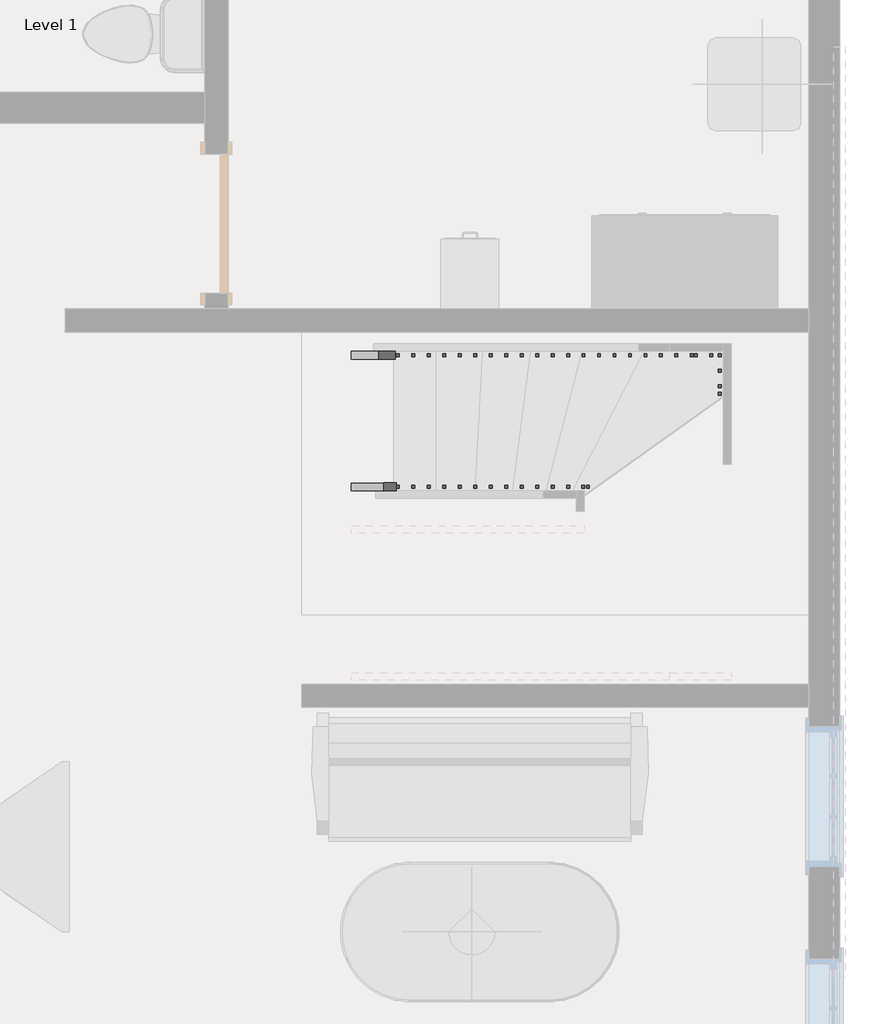
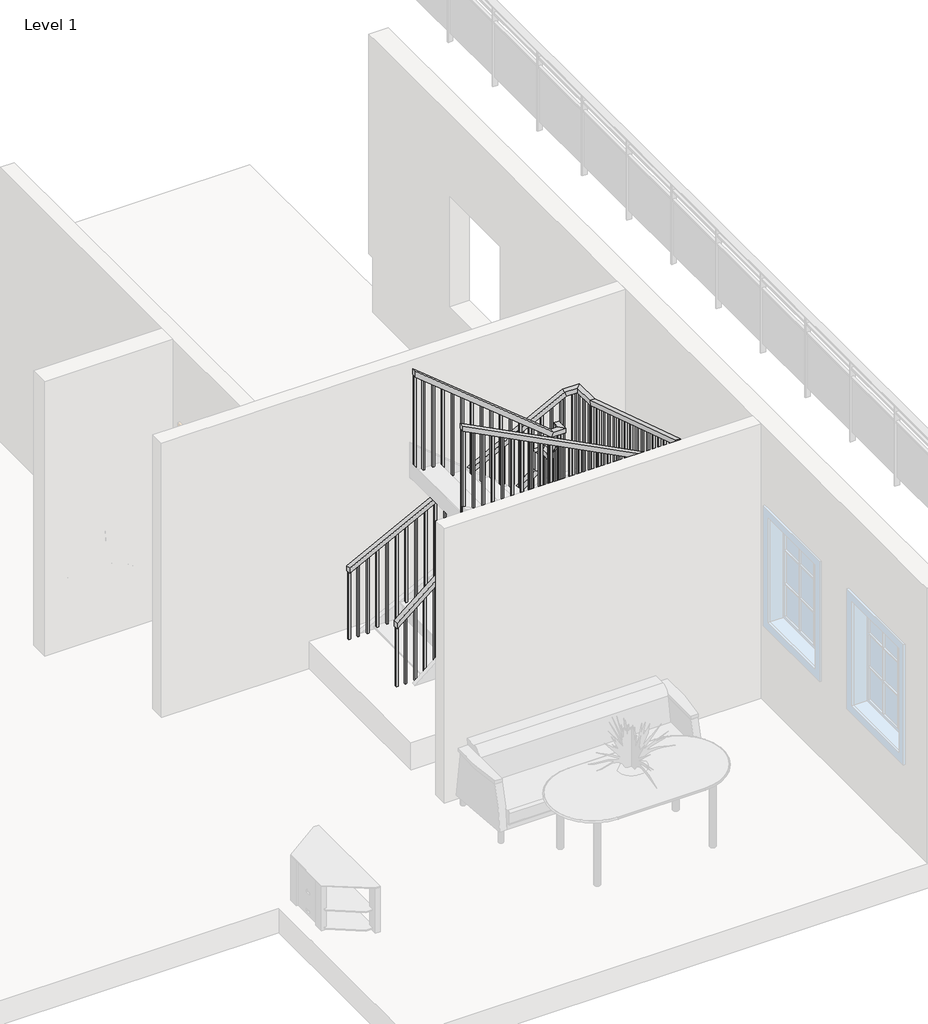
# One storey, part 2 of 4: 2 railings.
"""IFC4 building model written with IfcOpenShell, lengths in millimetres."""

from ifc_helpers import new_model, si_unit, frame, origin, place, context, project, spatial, polyline, outline, extrude, faceted_brep, element, save

model = new_model("IFC4")

# Units and contexts
model_context = context("Model", 3, world=origin())
ifc_project = project(units=[si_unit("LENGTHUNIT", "METRE", prefix="MILLI")], contexts=[model_context])

# Site, building, storey
site = spatial("IfcSite", under=ifc_project)
building = spatial("IfcBuilding", under=site)
storey = spatial("IfcBuildingStorey", under=building, Name="Level 1", Elevation=0.0)

# Railings
placement = place(None, origin())
element("IfcRailing", 1, ObjectType="Handrail - Rectangular", at=placement, inside=storey, context=model_context, shape_type="SolidModel", body=[
    faceted_brep([(-5316.1183874, 7519.8787933, 1025.2529681), (-5316.1183874, 7519.8787933, 959.7067088), (-5316.1183874, 7469.0787933, 959.7067088), (-5316.1183874, 7469.0787933, 1025.2529681), (-3864.5866955, 7519.8787933, 2208.7848338), (-3813.7866955, 7519.8787933, 2184.659247), (-3813.7866955, 7469.0787933, 2184.659247), (-3864.5866955, 7469.0787933, 2208.7848338), (-3864.5866955, 7519.8787933, 2414.6281882), (-3813.7866955, 7519.8787933, 2363.8281882), (-3813.7866955, 7469.0787933, 2363.8281882), (-3864.5866955, 7469.0787933, 2414.6281882), (-3737.5866955, 7519.8787933, 2414.6281882), (-3737.5866955, 7519.8787933, 2363.8281882), (-3788.3866955, 7469.0787933, 2363.8281882), (-3788.3866955, 7469.0787933, 2414.6281882), (-3737.5866955, 7392.8787933, 2414.6281882), (-3737.5866955, 7363.7574594, 2363.8281882), (-3788.3866955, 7363.7574594, 2363.8281882), (-3788.3866955, 7392.8787933, 2414.6281882), (-3737.5866955, 7265.8787933, 2631.5051451), (-3737.5866955, 7215.0787933, 2617.7256424), (-3788.3866955, 7215.0787933, 2617.7256424), (-3788.3866955, 7265.8787933, 2631.5051451), (-3737.5866955, 7265.8787933, 2837.3484995), (-3737.5866955, 7215.0787933, 2786.5484995), (-3788.3866955, 7215.0787933, 2786.5484995), (-3788.3866955, 7265.8787933, 2837.3484995), (-3737.5866955, 7138.8787933, 2837.3484995), (-3737.5866955, 7138.8787933, 2786.5484995), (-3788.3866955, 7189.6787933, 2786.5484995), (-3788.3866955, 7189.6787933, 2837.3484995), (-3864.5866955, 7138.8787933, 2837.3484995), (-3882.6721086, 7138.8787933, 2786.5484995), (-3882.6721086, 7189.6787933, 2786.5484995), (-3864.5866955, 7189.6787933, 2837.3484995), (-5316.1183874, 7138.8787933, 4020.8803652), (-5316.1183874, 7189.6787933, 4020.8803652), (-5316.1183874, 7189.6787933, 3955.3341059), (-5316.1183874, 7138.8787933, 3955.3341059)], [[[0, 1, 2, 3]], [[1, 0, 4, 5]], [[2, 1, 5, 6]], [[3, 2, 6, 7]], [[0, 3, 7, 4]], [[5, 4, 8, 9]], [[6, 5, 9, 10]], [[7, 6, 10, 11]], [[4, 7, 11, 8]], [[9, 8, 12, 13]], [[10, 9, 13, 14]], [[11, 10, 14, 15]], [[8, 11, 15, 12]], [[13, 12, 16, 17]], [[14, 13, 17, 18]], [[15, 14, 18, 19]], [[12, 15, 19, 16]], [[17, 16, 20, 21]], [[18, 17, 21, 22]], [[19, 18, 22, 23]], [[16, 19, 23, 20]], [[21, 20, 24, 25]], [[22, 21, 25, 26]], [[23, 22, 26, 27]], [[20, 23, 27, 24]], [[25, 24, 28, 29]], [[26, 25, 29, 30]], [[27, 26, 30, 31]], [[24, 27, 31, 28]], [[29, 28, 32, 33]], [[30, 29, 33, 34]], [[31, 30, 34, 35]], [[28, 31, 35, 32]], [[36, 37, 38, 39]], [[33, 32, 36, 39]], [[34, 33, 39, 38]], [[35, 34, 38, 37]], [[32, 35, 37, 36]]]),
    extrude(outline(polyline([(3866.2231262, -5206.8290519), (3881.7558784, -5225.8790519), (2878.6666667, -5225.8790519), (2878.6666667, -5206.8290519), (3866.2231262, -5206.8290519)])), frame((0.0, 7154.7537933, 0.0), z_axis=(0.0, 1.0, 0.0), x_axis=(0.0, 0.0, 1.0)), (0.0, 0.0, 1.0), 19.05),
    extrude(outline(polyline([(3783.3817813, -5105.2290519), (3798.9145334, -5124.2790519), (2878.6666667, -5124.2790519), (2878.6666667, -5105.2290519), (3783.3817813, -5105.2290519)])), frame((0.0, 7154.7537933, 0.0), z_axis=(0.0, 1.0, 0.0), x_axis=(0.0, 0.0, 1.0)), (0.0, 0.0, 1.0), 19.05),
    extrude(outline(polyline([(3700.5404364, -5003.6290519), (3716.0731885, -5022.6790519), (2709.3333333, -5022.6790519), (2709.3333333, -5003.6290519), (3700.5404364, -5003.6290519)])), frame((0.0, 7154.7537933, 0.0), z_axis=(0.0, 1.0, 0.0), x_axis=(0.0, 0.0, 1.0)), (0.0, 0.0, 1.0), 19.05),
    extrude(outline(polyline([(3617.6990914, -4902.0290519), (3633.2318436, -4921.0790519), (2709.3333333, -4921.0790519), (2709.3333333, -4902.0290519), (3617.6990914, -4902.0290519)])), frame((0.0, 7154.7537933, 0.0), z_axis=(0.0, 1.0, 0.0), x_axis=(0.0, 0.0, 1.0)), (0.0, 0.0, 1.0), 19.05),
    extrude(outline(polyline([(3534.8577465, -4800.4290519), (3550.3904987, -4819.4790519), (2709.3333333, -4819.4790519), (2709.3333333, -4800.4290519), (3534.8577465, -4800.4290519)])), frame((0.0, 7154.7537933, 0.0), z_axis=(0.0, 1.0, 0.0), x_axis=(0.0, 0.0, 1.0)), (0.0, 0.0, 1.0), 19.05),
    extrude(outline(polyline([(3452.0164016, -4698.8290519), (3467.5491538, -4717.8790519), (2540.0, -4717.8790519), (2540.0, -4698.8290519), (3452.0164016, -4698.8290519)])), frame((0.0, 7154.7537933, 0.0), z_axis=(0.0, 1.0, 0.0), x_axis=(0.0, 0.0, 1.0)), (0.0, 0.0, 1.0), 19.05),
    extrude(outline(polyline([(3369.1750567, -4597.2290519), (3384.7078088, -4616.2790519), (2540.0, -4616.2790519), (2540.0, -4597.2290519), (3369.1750567, -4597.2290519)])), frame((0.0, 7154.7537933, 0.0), z_axis=(0.0, 1.0, 0.0), x_axis=(0.0, 0.0, 1.0)), (0.0, 0.0, 1.0), 19.05),
    extrude(outline(polyline([(3286.3337117, -4495.6290519), (3301.8664639, -4514.6790519), (2540.0, -4514.6790519), (2540.0, -4495.6290519), (3286.3337117, -4495.6290519)])), frame((0.0, 7154.7537933, 0.0), z_axis=(0.0, 1.0, 0.0), x_axis=(0.0, 0.0, 1.0)), (0.0, 0.0, 1.0), 19.05),
    extrude(outline(polyline([(3203.4923668, -4394.0290519), (3219.025119, -4413.0790519), (2370.6666667, -4413.0790519), (2370.6666667, -4394.0290519), (3203.4923668, -4394.0290519)])), frame((0.0, 7154.7537933, 0.0), z_axis=(0.0, 1.0, 0.0), x_axis=(0.0, 0.0, 1.0)), (0.0, 0.0, 1.0), 19.05),
    extrude(outline(polyline([(3120.6510219, -4292.4290519), (3136.1837741, -4311.4790519), (2370.6666667, -4311.4790519), (2370.6666667, -4292.4290519), (3120.6510219, -4292.4290519)])), frame((0.0, 7154.7537933, 0.0), z_axis=(0.0, 1.0, 0.0), x_axis=(0.0, 0.0, 1.0)), (0.0, 0.0, 1.0), 19.05),
    extrude(outline(polyline([(3037.809677, -4190.8290519), (3053.3424291, -4209.8790519), (2201.3333333, -4209.8790519), (2201.3333333, -4190.8290519), (3037.809677, -4190.8290519)])), frame((0.0, 7154.7537933, 0.0), z_axis=(0.0, 1.0, 0.0), x_axis=(0.0, 0.0, 1.0)), (0.0, 0.0, 1.0), 19.05),
    extrude(outline(polyline([(2954.9683321, -4089.2290519), (2970.5010842, -4108.2790519), (2201.3333333, -4108.2790519), (2201.3333333, -4089.2290519), (2954.9683321, -4089.2290519)])), frame((0.0, 7154.7537933, 0.0), z_axis=(0.0, 1.0, 0.0), x_axis=(0.0, 0.0, 1.0)), (0.0, 0.0, 1.0), 19.05),
    extrude(outline(polyline([(2872.1269871, -3987.6290519), (2887.6597393, -4006.6790519), (2032.0, -4006.6790519), (2032.0, -3987.6290519), (2872.1269871, -3987.6290519)])), frame((0.0, 7154.7537933, 0.0), z_axis=(0.0, 1.0, 0.0), x_axis=(0.0, 0.0, 1.0)), (0.0, 0.0, 1.0), 19.05),
    extrude(outline(polyline([(2789.2856422, -3886.0290519), (2804.8183944, -3905.0790519), (2032.0, -3905.0790519), (2032.0, -3886.0290519), (2789.2856422, -3886.0290519)])), frame((0.0, 7154.7537933, 0.0), z_axis=(0.0, 1.0, 0.0), x_axis=(0.0, 0.0, 1.0)), (0.0, 0.0, 1.0), 19.05),
    extrude(outline(polyline([(7266.9678895, 2529.115018), (7286.0178895, 2496.5834745), (7286.0178895, 1524.0), (7266.9678895, 1524.0), (7266.9678895, 2529.115018)])), frame((-3772.5116955, 0.0, 0.0), z_axis=(1.0, 0.0, 0.0), x_axis=(0.0, 1.0, 0.0)), (0.0, 0.0, 1.0), 19.05),
    extrude(outline(polyline([(7368.5678895, 2355.6134525), (7387.6178895, 2323.0819089), (7387.6178895, 1524.0), (7368.5678895, 1524.0), (7368.5678895, 2355.6134525)])), frame((-3772.5116955, 0.0, 0.0), z_axis=(1.0, 0.0, 0.0), x_axis=(0.0, 1.0, 0.0)), (0.0, 0.0, 1.0), 19.05),
    extrude(outline(polyline([(2127.2519138, -3884.1933874), (2111.7191617, -3903.2433874), (1016.0, -3903.2433874), (1016.0, -3884.1933874), (2127.2519138, -3884.1933874)])), frame((0.0, 7484.9537933, 0.0), z_axis=(0.0, 1.0, 0.0), x_axis=(0.0, 0.0, 1.0)), (0.0, 0.0, 1.0), 19.05),
    extrude(outline(polyline([(2044.4105689, -3985.7933874), (2028.8778167, -4004.8433874), (1016.0, -4004.8433874), (1016.0, -3985.7933874), (2044.4105689, -3985.7933874)])), frame((0.0, 7484.9537933, 0.0), z_axis=(0.0, 1.0, 0.0), x_axis=(0.0, 0.0, 1.0)), (0.0, 0.0, 1.0), 19.05),
    extrude(outline(polyline([(1961.569224, -4087.3933874), (1946.0364718, -4106.4433874), (846.6666667, -4106.4433874), (846.6666667, -4087.3933874), (1961.569224, -4087.3933874)])), frame((0.0, 7484.9537933, 0.0), z_axis=(0.0, 1.0, 0.0), x_axis=(0.0, 0.0, 1.0)), (0.0, 0.0, 1.0), 19.05),
    extrude(outline(polyline([(1878.7278791, -4188.9933874), (1863.1951269, -4208.0433874), (846.6666667, -4208.0433874), (846.6666667, -4188.9933874), (1878.7278791, -4188.9933874)])), frame((0.0, 7484.9537933, 0.0), z_axis=(0.0, 1.0, 0.0), x_axis=(0.0, 0.0, 1.0)), (0.0, 0.0, 1.0), 19.05),
    extrude(outline(polyline([(1795.8865341, -4290.5933874), (1780.353782, -4309.6433874), (677.3333333, -4309.6433874), (677.3333333, -4290.5933874), (1795.8865341, -4290.5933874)])), frame((0.0, 7484.9537933, 0.0), z_axis=(0.0, 1.0, 0.0), x_axis=(0.0, 0.0, 1.0)), (0.0, 0.0, 1.0), 19.05),
    extrude(outline(polyline([(1713.0451892, -4392.1933874), (1697.5124371, -4411.2433874), (677.3333333, -4411.2433874), (677.3333333, -4392.1933874), (1713.0451892, -4392.1933874)])), frame((0.0, 7484.9537933, 0.0), z_axis=(0.0, 1.0, 0.0), x_axis=(0.0, 0.0, 1.0)), (0.0, 0.0, 1.0), 19.05),
    extrude(outline(polyline([(1630.2038443, -4493.7933874), (1614.6710921, -4512.8433874), (508.0, -4512.8433874), (508.0, -4493.7933874), (1630.2038443, -4493.7933874)])), frame((0.0, 7484.9537933, 0.0), z_axis=(0.0, 1.0, 0.0), x_axis=(0.0, 0.0, 1.0)), (0.0, 0.0, 1.0), 19.05),
    extrude(outline(polyline([(1547.3624994, -4595.3933874), (1531.8297472, -4614.4433874), (508.0, -4614.4433874), (508.0, -4595.3933874), (1547.3624994, -4595.3933874)])), frame((0.0, 7484.9537933, 0.0), z_axis=(0.0, 1.0, 0.0), x_axis=(0.0, 0.0, 1.0)), (0.0, 0.0, 1.0), 19.05),
    extrude(outline(polyline([(1464.5211545, -4696.9933874), (1448.9884023, -4716.0433874), (508.0, -4716.0433874), (508.0, -4696.9933874), (1464.5211545, -4696.9933874)])), frame((0.0, 7484.9537933, 0.0), z_axis=(0.0, 1.0, 0.0), x_axis=(0.0, 0.0, 1.0)), (0.0, 0.0, 1.0), 19.05),
    extrude(outline(polyline([(1381.6798095, -4798.5933874), (1366.1470574, -4817.6433874), (338.6666667, -4817.6433874), (338.6666667, -4798.5933874), (1381.6798095, -4798.5933874)])), frame((0.0, 7484.9537933, 0.0), z_axis=(0.0, 1.0, 0.0), x_axis=(0.0, 0.0, 1.0)), (0.0, 0.0, 1.0), 19.05),
    extrude(outline(polyline([(1298.8384646, -4900.1933874), (1283.3057124, -4919.2433874), (338.6666667, -4919.2433874), (338.6666667, -4900.1933874), (1298.8384646, -4900.1933874)])), frame((0.0, 7484.9537933, 0.0), z_axis=(0.0, 1.0, 0.0), x_axis=(0.0, 0.0, 1.0)), (0.0, 0.0, 1.0), 19.05),
    extrude(outline(polyline([(1215.9971197, -5001.7933874), (1200.4643675, -5020.8433874), (338.6666667, -5020.8433874), (338.6666667, -5001.7933874), (1215.9971197, -5001.7933874)])), frame((0.0, 7484.9537933, 0.0), z_axis=(0.0, 1.0, 0.0), x_axis=(0.0, 0.0, 1.0)), (0.0, 0.0, 1.0), 19.05),
    extrude(outline(polyline([(1133.1557748, -5103.3933874), (1117.6230226, -5122.4433874), (169.3333333, -5122.4433874), (169.3333333, -5103.3933874), (1133.1557748, -5103.3933874)])), frame((0.0, 7484.9537933, 0.0), z_axis=(0.0, 1.0, 0.0), x_axis=(0.0, 0.0, 1.0)), (0.0, 0.0, 1.0), 19.05),
    extrude(outline(polyline([(1050.3144298, -5204.9933874), (1034.7816777, -5224.0433874), (169.3333333, -5224.0433874), (169.3333333, -5204.9933874), (1050.3144298, -5204.9933874)])), frame((0.0, 7484.9537933, 0.0), z_axis=(0.0, 1.0, 0.0), x_axis=(0.0, 0.0, 1.0)), (0.0, 0.0, 1.0), 19.05),
    extrude(outline(polyline([(-3784.4290519, 7173.8037933), (-3784.4290519, 7154.7537933), (-3803.4790519, 7154.7537933), (-3803.4790519, 7173.8037933), (-3784.4290519, 7173.8037933)])), frame((0.0, 0.0, 1862.6666667), z_axis=(0.0, 0.0, 1.0), x_axis=(1.0, 0.0, 0.0)), (0.0, 0.0, 1.0), 923.8818329),
    extrude(outline(polyline([(-3772.5116955, 7173.8037933), (-3753.4616955, 7173.8037933), (-3753.4616955, 7154.7537933), (-3772.5116955, 7154.7537933), (-3772.5116955, 7173.8037933)])), frame((0.0, 0.0, 1862.6666667), z_axis=(0.0, 0.0, 1.0), x_axis=(1.0, 0.0, 0.0)), (0.0, 0.0, 1.0), 923.8818329),
    extrude(outline(polyline([(-3772.5116955, 7188.589697), (-3753.4616955, 7188.589697), (-3753.4616955, 7169.539697), (-3772.5116955, 7169.539697), (-3772.5116955, 7188.589697)])), frame((0.0, 0.0, 1693.3333333), z_axis=(0.0, 0.0, 1.0), x_axis=(1.0, 0.0, 0.0)), (0.0, 0.0, 1.0), 1093.2151662),
    extrude(outline(polyline([(-3772.5116955, 7489.2178895), (-3753.4616955, 7489.2178895), (-3753.4616955, 7470.1678895), (-3772.5116955, 7470.1678895), (-3772.5116955, 7489.2178895)])), frame((0.0, 0.0, 1354.6666667), z_axis=(0.0, 0.0, 1.0), x_axis=(1.0, 0.0, 0.0)), (0.0, 0.0, 1.0), 1009.1615215),
    extrude(outline(polyline([(-3772.5116955, 7484.9537933), (-3772.5116955, 7504.0037933), (-3753.4616955, 7504.0037933), (-3753.4616955, 7484.9537933), (-3772.5116955, 7484.9537933)])), frame((0.0, 0.0, 1185.3333333), z_axis=(0.0, 0.0, 1.0), x_axis=(1.0, 0.0, 0.0)), (0.0, 0.0, 1.0), 1178.4948549),
    extrude(outline(polyline([(-3803.4790519, 7484.9537933), (-3803.4790519, 7504.0037933), (-3784.4290519, 7504.0037933), (-3784.4290519, 7484.9537933), (-3803.4790519, 7484.9537933)])), frame((0.0, 0.0, 1185.3333333), z_axis=(0.0, 0.0, 1.0), x_axis=(1.0, 0.0, 0.0)), (0.0, 0.0, 1.0), 1178.4948549),
    extrude(outline(polyline([(3939.8013537, -5297.0683874), (3955.3341059, -5316.1183874), (2878.6666667, -5316.1183874), (2878.6666667, -5297.0683874), (3939.8013537, -5297.0683874)])), frame((0.0, 7154.7537933, 0.0), z_axis=(0.0, 1.0, 0.0), x_axis=(0.0, 0.0, 1.0)), (0.0, 0.0, 1.0), 19.05),
    extrude(outline(polyline([(975.239461, -5297.0683874), (959.7067088, -5316.1183874), (169.3333333, -5316.1183874), (169.3333333, -5297.0683874), (975.239461, -5297.0683874)])), frame((0.0, 7484.9537933, 0.0), z_axis=(0.0, 1.0, 0.0), x_axis=(0.0, 0.0, 1.0)), (0.0, 0.0, 1.0), 19.05),
])
element("IfcRailing", 2, ObjectType="Handrail - Rectangular", at=placement, inside=storey, context=model_context, shape_type="SolidModel", body=[
    faceted_brep([(-5316.1183874, 8383.4787933, 1109.0771751), (-5316.1183874, 8383.4787933, 1051.9280057), (-5316.1183874, 8332.6787933, 1051.9280057), (-5316.1183874, 8332.6787933, 1109.0771751), (-3056.1365309, 8383.4787933, 2273.7644996), (-3043.8164796, 8383.4787933, 2222.9644996), (-3043.8164796, 8332.6787933, 2222.9644996), (-3056.1365309, 8332.6787933, 2273.7644996), (-2873.9866955, 8383.4787933, 2273.7644996), (-2873.9866955, 8383.4787933, 2222.9644996), (-2924.7866955, 8332.6787933, 2222.9644996), (-2924.7866955, 8332.6787933, 2273.7644996), (-2873.9866955, 8106.3248407, 2273.7644996), (-2873.9866955, 8098.3742645, 2222.9644996), (-2924.7866955, 8098.3742645, 2222.9644996), (-2924.7866955, 8106.3248407, 2273.7644996), (-2873.9866955, 6552.4327459, 2772.3688337), (-2873.9866955, 6544.4821698, 2721.5688337), (-2924.7866955, 6544.4821698, 2721.5688337), (-2924.7866955, 6552.4327459, 2772.3688337), (-2873.9866955, 6275.2787933, 2772.3688337), (-2873.9866955, 6275.2787933, 2721.5688337), (-2924.7866955, 6326.0787933, 2721.5688337), (-2924.7866955, 6326.0787933, 2772.3688337), (-3056.1365309, 6275.2787933, 2772.3688337), (-3068.4565822, 6275.2787933, 2721.5688337), (-3068.4565822, 6326.0787933, 2721.5688337), (-3056.1365309, 6326.0787933, 2772.3688337), (-5316.1183874, 6275.2787933, 3937.0561582), (-5316.1183874, 6326.0787933, 3937.0561582), (-5316.1183874, 6326.0787933, 3879.9069889), (-5316.1183874, 6275.2787933, 3879.9069889)], [[[0, 1, 2, 3]], [[1, 0, 4, 5]], [[2, 1, 5, 6]], [[3, 2, 6, 7]], [[0, 3, 7, 4]], [[5, 4, 8, 9]], [[6, 5, 9, 10]], [[7, 6, 10, 11]], [[4, 7, 11, 8]], [[9, 8, 12, 13]], [[10, 9, 13, 14]], [[11, 10, 14, 15]], [[8, 11, 15, 12]], [[13, 12, 16, 17]], [[14, 13, 17, 18]], [[15, 14, 18, 19]], [[12, 15, 19, 16]], [[17, 16, 20, 21]], [[18, 17, 21, 22]], [[19, 18, 22, 23]], [[16, 19, 23, 20]], [[21, 20, 24, 25]], [[22, 21, 25, 26]], [[23, 22, 26, 27]], [[20, 23, 27, 24]], [[28, 29, 30, 31]], [[25, 24, 28, 31]], [[26, 25, 31, 30]], [[27, 26, 30, 29]], [[24, 27, 29, 28]]]),
    extrude(outline(polyline([(3872.0443296, -5300.8615309), (2878.6666667, -5300.8615309), (2878.6666667, -5281.8115309), (3862.2268642, -5281.8115309), (3872.0443296, -5300.8615309)])), frame((0.0, 6291.1537933, 0.0), z_axis=(0.0, 1.0, 0.0), x_axis=(0.0, 0.0, 1.0)), (0.0, 0.0, 1.0), 19.05),
    extrude(outline(polyline([(3819.6845145, -5199.2615309), (2878.6666667, -5199.2615309), (2878.6666667, -5180.2115309), (3809.8670491, -5180.2115309), (3819.6845145, -5199.2615309)])), frame((0.0, 6291.1537933, 0.0), z_axis=(0.0, 1.0, 0.0), x_axis=(0.0, 0.0, 1.0)), (0.0, 0.0, 1.0), 19.05),
    extrude(outline(polyline([(3767.3246993, -5097.6615309), (2878.6666667, -5097.6615309), (2878.6666667, -5078.6115309), (3757.507234, -5078.6115309), (3767.3246993, -5097.6615309)])), frame((0.0, 6291.1537933, 0.0), z_axis=(0.0, 1.0, 0.0), x_axis=(0.0, 0.0, 1.0)), (0.0, 0.0, 1.0), 19.05),
    extrude(outline(polyline([(3714.9648842, -4996.0615309), (2709.3333333, -4996.0615309), (2709.3333333, -4977.0115309), (3705.1474189, -4977.0115309), (3714.9648842, -4996.0615309)])), frame((0.0, 6291.1537933, 0.0), z_axis=(0.0, 1.0, 0.0), x_axis=(0.0, 0.0, 1.0)), (0.0, 0.0, 1.0), 19.05),
    extrude(outline(polyline([(3662.6050691, -4894.4615309), (2709.3333333, -4894.4615309), (2709.3333333, -4875.4115309), (3652.7876038, -4875.4115309), (3662.6050691, -4894.4615309)])), frame((0.0, 6291.1537933, 0.0), z_axis=(0.0, 1.0, 0.0), x_axis=(0.0, 0.0, 1.0)), (0.0, 0.0, 1.0), 19.05),
    extrude(outline(polyline([(3610.245254, -4792.8615309), (2709.3333333, -4792.8615309), (2709.3333333, -4773.8115309), (3600.4277887, -4773.8115309), (3610.245254, -4792.8615309)])), frame((0.0, 6291.1537933, 0.0), z_axis=(0.0, 1.0, 0.0), x_axis=(0.0, 0.0, 1.0)), (0.0, 0.0, 1.0), 19.05),
    extrude(outline(polyline([(3557.8854389, -4691.2615309), (2540.0, -4691.2615309), (2540.0, -4672.2115309), (3548.0679735, -4672.2115309), (3557.8854389, -4691.2615309)])), frame((0.0, 6291.1537933, 0.0), z_axis=(0.0, 1.0, 0.0), x_axis=(0.0, 0.0, 1.0)), (0.0, 0.0, 1.0), 19.05),
    extrude(outline(polyline([(3505.5256238, -4589.6615309), (2540.0, -4589.6615309), (2540.0, -4570.6115309), (3495.7081584, -4570.6115309), (3505.5256238, -4589.6615309)])), frame((0.0, 6291.1537933, 0.0), z_axis=(0.0, 1.0, 0.0), x_axis=(0.0, 0.0, 1.0)), (0.0, 0.0, 1.0), 19.05),
    extrude(outline(polyline([(3453.1658086, -4488.0615309), (2540.0, -4488.0615309), (2540.0, -4469.0115309), (3443.3483433, -4469.0115309), (3453.1658086, -4488.0615309)])), frame((0.0, 6291.1537933, 0.0), z_axis=(0.0, 1.0, 0.0), x_axis=(0.0, 0.0, 1.0)), (0.0, 0.0, 1.0), 19.05),
    extrude(outline(polyline([(3400.8059935, -4386.4615309), (2370.6666667, -4386.4615309), (2370.6666667, -4367.4115309), (3390.9885282, -4367.4115309), (3400.8059935, -4386.4615309)])), frame((0.0, 6291.1537933, 0.0), z_axis=(0.0, 1.0, 0.0), x_axis=(0.0, 0.0, 1.0)), (0.0, 0.0, 1.0), 19.05),
    extrude(outline(polyline([(3348.4461784, -4284.8615309), (2370.6666667, -4284.8615309), (2370.6666667, -4265.8115309), (3338.6287131, -4265.8115309), (3348.4461784, -4284.8615309)])), frame((0.0, 6291.1537933, 0.0), z_axis=(0.0, 1.0, 0.0), x_axis=(0.0, 0.0, 1.0)), (0.0, 0.0, 1.0), 19.05),
    extrude(outline(polyline([(3296.0863633, -4183.2615309), (2370.6666667, -4183.2615309), (2370.6666667, -4164.2115309), (3286.268898, -4164.2115309), (3296.0863633, -4183.2615309)])), frame((0.0, 6291.1537933, 0.0), z_axis=(0.0, 1.0, 0.0), x_axis=(0.0, 0.0, 1.0)), (0.0, 0.0, 1.0), 19.05),
    extrude(outline(polyline([(3243.7265482, -4081.6615309), (2201.3333333, -4081.6615309), (2201.3333333, -4062.6115309), (3233.9090828, -4062.6115309), (3243.7265482, -4081.6615309)])), frame((0.0, 6291.1537933, 0.0), z_axis=(0.0, 1.0, 0.0), x_axis=(0.0, 0.0, 1.0)), (0.0, 0.0, 1.0), 19.05),
    extrude(outline(polyline([(3191.3667331, -3980.0615309), (2201.3333333, -3980.0615309), (2201.3333333, -3961.0115309), (3181.5492677, -3961.0115309), (3191.3667331, -3980.0615309)])), frame((0.0, 6291.1537933, 0.0), z_axis=(0.0, 1.0, 0.0), x_axis=(0.0, 0.0, 1.0)), (0.0, 0.0, 1.0), 19.05),
    extrude(outline(polyline([(3139.0069179, -3878.4615309), (2201.3333333, -3878.4615309), (2201.3333333, -3859.4115309), (3129.1894526, -3859.4115309), (3139.0069179, -3878.4615309)])), frame((0.0, 6291.1537933, 0.0), z_axis=(0.0, 1.0, 0.0), x_axis=(0.0, 0.0, 1.0)), (0.0, 0.0, 1.0), 19.05),
    extrude(outline(polyline([(3086.6471028, -3776.8615309), (2032.0, -3776.8615309), (2032.0, -3757.8115309), (3076.8296375, -3757.8115309), (3086.6471028, -3776.8615309)])), frame((0.0, 6291.1537933, 0.0), z_axis=(0.0, 1.0, 0.0), x_axis=(0.0, 0.0, 1.0)), (0.0, 0.0, 1.0), 19.05),
    extrude(outline(polyline([(3034.2872877, -3675.2615309), (2032.0, -3675.2615309), (2032.0, -3656.2115309), (3024.4698224, -3656.2115309), (3034.2872877, -3675.2615309)])), frame((0.0, 6291.1537933, 0.0), z_axis=(0.0, 1.0, 0.0), x_axis=(0.0, 0.0, 1.0)), (0.0, 0.0, 1.0), 19.05),
    extrude(outline(polyline([(2981.9274726, -3573.6615309), (2032.0, -3573.6615309), (2032.0, -3554.6115309), (2972.1100073, -3554.6115309), (2981.9274726, -3573.6615309)])), frame((0.0, 6291.1537933, 0.0), z_axis=(0.0, 1.0, 0.0), x_axis=(0.0, 0.0, 1.0)), (0.0, 0.0, 1.0), 19.05),
    extrude(outline(polyline([(2929.5676575, -3472.0615309), (2032.0, -3472.0615309), (2032.0, -3453.0115309), (2919.7501921, -3453.0115309), (2929.5676575, -3472.0615309)])), frame((0.0, 6291.1537933, 0.0), z_axis=(0.0, 1.0, 0.0), x_axis=(0.0, 0.0, 1.0)), (0.0, 0.0, 1.0), 19.05),
    extrude(outline(polyline([(2877.2078424, -3370.4615309), (1862.6666667, -3370.4615309), (1862.6666667, -3351.4115309), (2867.390377, -3351.4115309), (2877.2078424, -3370.4615309)])), frame((0.0, 6291.1537933, 0.0), z_axis=(0.0, 1.0, 0.0), x_axis=(0.0, 0.0, 1.0)), (0.0, 0.0, 1.0), 19.05),
    extrude(outline(polyline([(2824.8480272, -3268.8615309), (1862.6666667, -3268.8615309), (1862.6666667, -3249.8115309), (2815.0305619, -3249.8115309), (2824.8480272, -3268.8615309)])), frame((0.0, 6291.1537933, 0.0), z_axis=(0.0, 1.0, 0.0), x_axis=(0.0, 0.0, 1.0)), (0.0, 0.0, 1.0), 19.05),
    extrude(outline(polyline([(2772.4882121, -3167.2615309), (1862.6666667, -3167.2615309), (1862.6666667, -3148.2115309), (2762.6707468, -3148.2115309), (2772.4882121, -3167.2615309)])), frame((0.0, 6291.1537933, 0.0), z_axis=(0.0, 1.0, 0.0), x_axis=(0.0, 0.0, 1.0)), (0.0, 0.0, 1.0), 19.05),
    extrude(outline(polyline([(-2991.4616955, 6291.1537933), (-3010.5116955, 6291.1537933), (-3010.5116955, 6310.2037933), (-2991.4616955, 6310.2037933), (-2991.4616955, 6291.1537933)])), frame((0.0, 0.0, 1862.6666667), z_axis=(0.0, 0.0, 1.0), x_axis=(1.0, 0.0, 0.0)), (0.0, 0.0, 1.0), 858.902167),
    extrude(outline(polyline([(-2889.8616955, 6358.7577459), (-2889.8616955, 6339.7077459), (-2908.9116955, 6339.7077459), (-2908.9116955, 6358.7577459), (-2889.8616955, 6358.7577459)])), frame((0.0, 0.0, 1862.6666667), z_axis=(0.0, 0.0, 1.0), x_axis=(1.0, 0.0, 0.0)), (0.0, 0.0, 1.0), 858.902167),
    extrude(outline(polyline([(-2889.8616955, 6460.3577459), (-2889.8616955, 6441.3077459), (-2908.9116955, 6441.3077459), (-2908.9116955, 6460.3577459), (-2889.8616955, 6460.3577459)])), frame((0.0, 0.0, 1862.6666667), z_axis=(0.0, 0.0, 1.0), x_axis=(1.0, 0.0, 0.0)), (0.0, 0.0, 1.0), 858.902167),
    extrude(outline(polyline([(6591.8498407, 2706.3697564), (6591.8498407, 1693.3333333), (6572.7998407, 1693.3333333), (6572.7998407, 2712.4824155), (6591.8498407, 2706.3697564)])), frame((-2908.9116955, 0.0, 0.0), z_axis=(1.0, 0.0, 0.0), x_axis=(0.0, 1.0, 0.0)), (0.0, 0.0, 1.0), 19.05),
    extrude(outline(polyline([(6693.4498407, 2673.7689082), (6693.4498407, 1693.3333333), (6674.3998407, 1693.3333333), (6674.3998407, 2679.8815673), (6693.4498407, 2673.7689082)])), frame((-2908.9116955, 0.0, 0.0), z_axis=(1.0, 0.0, 0.0), x_axis=(0.0, 1.0, 0.0)), (0.0, 0.0, 1.0), 19.05),
    extrude(outline(polyline([(6795.0498407, 2641.16806), (6795.0498407, 1693.3333333), (6775.9998407, 1693.3333333), (6775.9998407, 2647.280719), (6795.0498407, 2641.16806)])), frame((-2908.9116955, 0.0, 0.0), z_axis=(1.0, 0.0, 0.0), x_axis=(0.0, 1.0, 0.0)), (0.0, 0.0, 1.0), 19.05),
    extrude(outline(polyline([(6896.6498407, 2608.5672118), (6896.6498407, 1693.3333333), (6877.5998407, 1693.3333333), (6877.5998407, 2614.6798708), (6896.6498407, 2608.5672118)])), frame((-2908.9116955, 0.0, 0.0), z_axis=(1.0, 0.0, 0.0), x_axis=(0.0, 1.0, 0.0)), (0.0, 0.0, 1.0), 19.05),
    extrude(outline(polyline([(6998.2498407, 2575.9663635), (6998.2498407, 1693.3333333), (6979.1998407, 1693.3333333), (6979.1998407, 2582.0790226), (6998.2498407, 2575.9663635)])), frame((-2908.9116955, 0.0, 0.0), z_axis=(1.0, 0.0, 0.0), x_axis=(0.0, 1.0, 0.0)), (0.0, 0.0, 1.0), 19.05),
    extrude(outline(polyline([(7099.8498407, 2543.3655153), (7099.8498407, 1693.3333333), (7080.7998407, 1693.3333333), (7080.7998407, 2549.4781744), (7099.8498407, 2543.3655153)])), frame((-2908.9116955, 0.0, 0.0), z_axis=(1.0, 0.0, 0.0), x_axis=(0.0, 1.0, 0.0)), (0.0, 0.0, 1.0), 19.05),
    extrude(outline(polyline([(7201.4498407, 2510.7646671), (7201.4498407, 1524.0), (7182.3998407, 1524.0), (7182.3998407, 2516.8773261), (7201.4498407, 2510.7646671)])), frame((-2908.9116955, 0.0, 0.0), z_axis=(1.0, 0.0, 0.0), x_axis=(0.0, 1.0, 0.0)), (0.0, 0.0, 1.0), 19.05),
    extrude(outline(polyline([(7303.0498407, 2478.1638189), (7303.0498407, 1524.0), (7283.9998407, 1524.0), (7283.9998407, 2484.2764779), (7303.0498407, 2478.1638189)])), frame((-2908.9116955, 0.0, 0.0), z_axis=(1.0, 0.0, 0.0), x_axis=(0.0, 1.0, 0.0)), (0.0, 0.0, 1.0), 19.05),
    extrude(outline(polyline([(7404.6498407, 2445.5629706), (7404.6498407, 1524.0), (7385.5998407, 1524.0), (7385.5998407, 2451.6756297), (7404.6498407, 2445.5629706)])), frame((-2908.9116955, 0.0, 0.0), z_axis=(1.0, 0.0, 0.0), x_axis=(0.0, 1.0, 0.0)), (0.0, 0.0, 1.0), 19.05),
    extrude(outline(polyline([(7506.2498407, 2412.9621224), (7506.2498407, 1524.0), (7487.1998407, 1524.0), (7487.1998407, 2419.0747814), (7506.2498407, 2412.9621224)])), frame((-2908.9116955, 0.0, 0.0), z_axis=(1.0, 0.0, 0.0), x_axis=(0.0, 1.0, 0.0)), (0.0, 0.0, 1.0), 19.05),
    extrude(outline(polyline([(7607.8498407, 2380.3612742), (7607.8498407, 1354.6666667), (7588.7998407, 1354.6666667), (7588.7998407, 2386.4739332), (7607.8498407, 2380.3612742)])), frame((-2908.9116955, 0.0, 0.0), z_axis=(1.0, 0.0, 0.0), x_axis=(0.0, 1.0, 0.0)), (0.0, 0.0, 1.0), 19.05),
    extrude(outline(polyline([(7709.4498407, 2347.7604259), (7709.4498407, 1354.6666667), (7690.3998407, 1354.6666667), (7690.3998407, 2353.873085), (7709.4498407, 2347.7604259)])), frame((-2908.9116955, 0.0, 0.0), z_axis=(1.0, 0.0, 0.0), x_axis=(0.0, 1.0, 0.0)), (0.0, 0.0, 1.0), 19.05),
    extrude(outline(polyline([(7811.0498407, 2315.1595777), (7811.0498407, 1354.6666667), (7791.9998407, 1354.6666667), (7791.9998407, 2321.2722368), (7811.0498407, 2315.1595777)])), frame((-2908.9116955, 0.0, 0.0), z_axis=(1.0, 0.0, 0.0), x_axis=(0.0, 1.0, 0.0)), (0.0, 0.0, 1.0), 19.05),
    extrude(outline(polyline([(7912.6498407, 2282.5587295), (7912.6498407, 1354.6666667), (7893.5998407, 1354.6666667), (7893.5998407, 2288.6713885), (7912.6498407, 2282.5587295)])), frame((-2908.9116955, 0.0, 0.0), z_axis=(1.0, 0.0, 0.0), x_axis=(0.0, 1.0, 0.0)), (0.0, 0.0, 1.0), 19.05),
    extrude(outline(polyline([(8014.2498407, 2249.9578813), (8014.2498407, 1354.6666667), (7995.1998407, 1354.6666667), (7995.1998407, 2256.0705403), (8014.2498407, 2249.9578813)])), frame((-2908.9116955, 0.0, 0.0), z_axis=(1.0, 0.0, 0.0), x_axis=(0.0, 1.0, 0.0)), (0.0, 0.0, 1.0), 19.05),
    extrude(outline(polyline([(-2889.8616955, 8164.4037933), (-2889.8616955, 8145.3537933), (-2908.9116955, 8145.3537933), (-2908.9116955, 8164.4037933), (-2889.8616955, 8164.4037933)])), frame((0.0, 0.0, 1185.3333333), z_axis=(0.0, 0.0, 1.0), x_axis=(1.0, 0.0, 0.0)), (0.0, 0.0, 1.0), 1037.6311663),
    extrude(outline(polyline([(-2889.8616955, 8266.0037933), (-2889.8616955, 8246.9537933), (-2908.9116955, 8246.9537933), (-2908.9116955, 8266.0037933), (-2889.8616955, 8266.0037933)])), frame((0.0, 0.0, 1185.3333333), z_axis=(0.0, 0.0, 1.0), x_axis=(1.0, 0.0, 0.0)), (0.0, 0.0, 1.0), 1037.6311663),
    extrude(outline(polyline([(-2964.0615309, 8367.6037933), (-2945.0115309, 8367.6037933), (-2945.0115309, 8348.5537933), (-2964.0615309, 8348.5537933), (-2964.0615309, 8367.6037933)])), frame((0.0, 0.0, 1185.3333333), z_axis=(0.0, 0.0, 1.0), x_axis=(1.0, 0.0, 0.0)), (0.0, 0.0, 1.0), 1037.6311663),
    extrude(outline(polyline([(2198.9352056, -3090.4433874), (1185.3333333, -3090.4433874), (1185.3333333, -3071.3933874), (2208.752671, -3071.3933874), (2198.9352056, -3090.4433874)])), frame((0.0, 8348.5537933, 0.0), z_axis=(0.0, 1.0, 0.0), x_axis=(0.0, 0.0, 1.0)), (0.0, 0.0, 1.0), 19.05),
    extrude(outline(polyline([(2146.5753905, -3192.0433874), (1185.3333333, -3192.0433874), (1185.3333333, -3172.9933874), (2156.3928558, -3172.9933874), (2146.5753905, -3192.0433874)])), frame((0.0, 8348.5537933, 0.0), z_axis=(0.0, 1.0, 0.0), x_axis=(0.0, 0.0, 1.0)), (0.0, 0.0, 1.0), 19.05),
    extrude(outline(polyline([(2094.2155754, -3293.6433874), (1185.3333333, -3293.6433874), (1185.3333333, -3274.5933874), (2104.0330407, -3274.5933874), (2094.2155754, -3293.6433874)])), frame((0.0, 8348.5537933, 0.0), z_axis=(0.0, 1.0, 0.0), x_axis=(0.0, 0.0, 1.0)), (0.0, 0.0, 1.0), 19.05),
    extrude(outline(polyline([(2041.8557603, -3395.2433874), (1185.3333333, -3395.2433874), (1185.3333333, -3376.1933874), (2051.6732256, -3376.1933874), (2041.8557603, -3395.2433874)])), frame((0.0, 8348.5537933, 0.0), z_axis=(0.0, 1.0, 0.0), x_axis=(0.0, 0.0, 1.0)), (0.0, 0.0, 1.0), 19.05),
    extrude(outline(polyline([(1989.4959452, -3496.8433874), (1016.0, -3496.8433874), (1016.0, -3477.7933874), (1999.3134105, -3477.7933874), (1989.4959452, -3496.8433874)])), frame((0.0, 8348.5537933, 0.0), z_axis=(0.0, 1.0, 0.0), x_axis=(0.0, 0.0, 1.0)), (0.0, 0.0, 1.0), 19.05),
    extrude(outline(polyline([(1937.13613, -3598.4433874), (1016.0, -3598.4433874), (1016.0, -3579.3933874), (1946.9535954, -3579.3933874), (1937.13613, -3598.4433874)])), frame((0.0, 8348.5537933, 0.0), z_axis=(0.0, 1.0, 0.0), x_axis=(0.0, 0.0, 1.0)), (0.0, 0.0, 1.0), 19.05),
    extrude(outline(polyline([(1884.7763149, -3700.0433874), (1016.0, -3700.0433874), (1016.0, -3680.9933874), (1894.5937803, -3680.9933874), (1884.7763149, -3700.0433874)])), frame((0.0, 8348.5537933, 0.0), z_axis=(0.0, 1.0, 0.0), x_axis=(0.0, 0.0, 1.0)), (0.0, 0.0, 1.0), 19.05),
    extrude(outline(polyline([(1832.4164998, -3801.6433874), (1016.0, -3801.6433874), (1016.0, -3782.5933874), (1842.2339651, -3782.5933874), (1832.4164998, -3801.6433874)])), frame((0.0, 8348.5537933, 0.0), z_axis=(0.0, 1.0, 0.0), x_axis=(0.0, 0.0, 1.0)), (0.0, 0.0, 1.0), 19.05),
    extrude(outline(polyline([(1780.0566847, -3903.2433874), (846.6666667, -3903.2433874), (846.6666667, -3884.1933874), (1789.87415, -3884.1933874), (1780.0566847, -3903.2433874)])), frame((0.0, 8348.5537933, 0.0), z_axis=(0.0, 1.0, 0.0), x_axis=(0.0, 0.0, 1.0)), (0.0, 0.0, 1.0), 19.05),
    extrude(outline(polyline([(1727.6968696, -4004.8433874), (846.6666667, -4004.8433874), (846.6666667, -3985.7933874), (1737.5143349, -3985.7933874), (1727.6968696, -4004.8433874)])), frame((0.0, 8348.5537933, 0.0), z_axis=(0.0, 1.0, 0.0), x_axis=(0.0, 0.0, 1.0)), (0.0, 0.0, 1.0), 19.05),
    extrude(outline(polyline([(1675.3370545, -4106.4433874), (846.6666667, -4106.4433874), (846.6666667, -4087.3933874), (1685.1545198, -4087.3933874), (1675.3370545, -4106.4433874)])), frame((0.0, 8348.5537933, 0.0), z_axis=(0.0, 1.0, 0.0), x_axis=(0.0, 0.0, 1.0)), (0.0, 0.0, 1.0), 19.05),
    extrude(outline(polyline([(1622.9772393, -4208.0433874), (677.3333333, -4208.0433874), (677.3333333, -4188.9933874), (1632.7947047, -4188.9933874), (1622.9772393, -4208.0433874)])), frame((0.0, 8348.5537933, 0.0), z_axis=(0.0, 1.0, 0.0), x_axis=(0.0, 0.0, 1.0)), (0.0, 0.0, 1.0), 19.05),
    extrude(outline(polyline([(1570.6174242, -4309.6433874), (677.3333333, -4309.6433874), (677.3333333, -4290.5933874), (1580.4348896, -4290.5933874), (1570.6174242, -4309.6433874)])), frame((0.0, 8348.5537933, 0.0), z_axis=(0.0, 1.0, 0.0), x_axis=(0.0, 0.0, 1.0)), (0.0, 0.0, 1.0), 19.05),
    extrude(outline(polyline([(1518.2576091, -4411.2433874), (677.3333333, -4411.2433874), (677.3333333, -4392.1933874), (1528.0750744, -4392.1933874), (1518.2576091, -4411.2433874)])), frame((0.0, 8348.5537933, 0.0), z_axis=(0.0, 1.0, 0.0), x_axis=(0.0, 0.0, 1.0)), (0.0, 0.0, 1.0), 19.05),
    extrude(outline(polyline([(1465.897794, -4512.8433874), (508.0, -4512.8433874), (508.0, -4493.7933874), (1475.7152593, -4493.7933874), (1465.897794, -4512.8433874)])), frame((0.0, 8348.5537933, 0.0), z_axis=(0.0, 1.0, 0.0), x_axis=(0.0, 0.0, 1.0)), (0.0, 0.0, 1.0), 19.05),
    extrude(outline(polyline([(1413.5379789, -4614.4433874), (508.0, -4614.4433874), (508.0, -4595.3933874), (1423.3554442, -4595.3933874), (1413.5379789, -4614.4433874)])), frame((0.0, 8348.5537933, 0.0), z_axis=(0.0, 1.0, 0.0), x_axis=(0.0, 0.0, 1.0)), (0.0, 0.0, 1.0), 19.05),
    extrude(outline(polyline([(1361.1781638, -4716.0433874), (508.0, -4716.0433874), (508.0, -4696.9933874), (1370.9956291, -4696.9933874), (1361.1781638, -4716.0433874)])), frame((0.0, 8348.5537933, 0.0), z_axis=(0.0, 1.0, 0.0), x_axis=(0.0, 0.0, 1.0)), (0.0, 0.0, 1.0), 19.05),
    extrude(outline(polyline([(1308.8183486, -4817.6433874), (338.6666667, -4817.6433874), (338.6666667, -4798.5933874), (1318.635814, -4798.5933874), (1308.8183486, -4817.6433874)])), frame((0.0, 8348.5537933, 0.0), z_axis=(0.0, 1.0, 0.0), x_axis=(0.0, 0.0, 1.0)), (0.0, 0.0, 1.0), 19.05),
    extrude(outline(polyline([(1256.4585335, -4919.2433874), (338.6666667, -4919.2433874), (338.6666667, -4900.1933874), (1266.2759989, -4900.1933874), (1256.4585335, -4919.2433874)])), frame((0.0, 8348.5537933, 0.0), z_axis=(0.0, 1.0, 0.0), x_axis=(0.0, 0.0, 1.0)), (0.0, 0.0, 1.0), 19.05),
    extrude(outline(polyline([(1204.0987184, -5020.8433874), (338.6666667, -5020.8433874), (338.6666667, -5001.7933874), (1213.9161837, -5001.7933874), (1204.0987184, -5020.8433874)])), frame((0.0, 8348.5537933, 0.0), z_axis=(0.0, 1.0, 0.0), x_axis=(0.0, 0.0, 1.0)), (0.0, 0.0, 1.0), 19.05),
    extrude(outline(polyline([(1151.7389033, -5122.4433874), (169.3333333, -5122.4433874), (169.3333333, -5103.3933874), (1161.5563686, -5103.3933874), (1151.7389033, -5122.4433874)])), frame((0.0, 8348.5537933, 0.0), z_axis=(0.0, 1.0, 0.0), x_axis=(0.0, 0.0, 1.0)), (0.0, 0.0, 1.0), 19.05),
    extrude(outline(polyline([(1099.3790882, -5224.0433874), (169.3333333, -5224.0433874), (169.3333333, -5204.9933874), (1109.1965535, -5204.9933874), (1099.3790882, -5224.0433874)])), frame((0.0, 8348.5537933, 0.0), z_axis=(0.0, 1.0, 0.0), x_axis=(0.0, 0.0, 1.0)), (0.0, 0.0, 1.0), 19.05),
    extrude(outline(polyline([(-3046.6115309, 6291.1537933), (-3065.6615309, 6291.1537933), (-3065.6615309, 6310.2037933), (-3046.6115309, 6310.2037933), (-3046.6115309, 6291.1537933)])), frame((0.0, 0.0, 1862.6666667), z_axis=(0.0, 0.0, 1.0), x_axis=(1.0, 0.0, 0.0)), (0.0, 0.0, 1.0), 858.902167),
    extrude(outline(polyline([(-2889.8616955, 6310.2037933), (-2889.8616955, 6291.1537933), (-2908.9116955, 6291.1537933), (-2908.9116955, 6310.2037933), (-2889.8616955, 6310.2037933)])), frame((0.0, 0.0, 1862.6666667), z_axis=(0.0, 0.0, 1.0), x_axis=(1.0, 0.0, 0.0)), (0.0, 0.0, 1.0), 858.902167),
    extrude(outline(polyline([(6561.9577459, 2715.9613671), (6561.9577459, 1862.6666667), (6542.9077459, 1862.6666667), (6542.9077459, 2722.0740262), (6561.9577459, 2715.9613671)])), frame((-2908.9116955, 0.0, 0.0), z_axis=(1.0, 0.0, 0.0), x_axis=(0.0, 1.0, 0.0)), (0.0, 0.0, 1.0), 19.05),
    extrude(outline(polyline([(-2889.8616955, 8115.8498407), (-2889.8616955, 8096.7998407), (-2908.9116955, 8096.7998407), (-2908.9116955, 8115.8498407), (-2889.8616955, 8115.8498407)])), frame((0.0, 0.0, 1185.3333333), z_axis=(0.0, 0.0, 1.0), x_axis=(1.0, 0.0, 0.0)), (0.0, 0.0, 1.0), 1037.6311663),
    extrude(outline(polyline([(-2908.9116955, 8367.6037933), (-2889.8616955, 8367.6037933), (-2889.8616955, 8348.5537933), (-2908.9116955, 8348.5537933), (-2908.9116955, 8367.6037933)])), frame((0.0, 0.0, 1185.3333333), z_axis=(0.0, 0.0, 1.0), x_axis=(1.0, 0.0, 0.0)), (0.0, 0.0, 1.0), 1037.6311663),
    extrude(outline(polyline([(2211.7065976, -3065.6615309), (1185.3333333, -3065.6615309), (1185.3333333, -3046.6115309), (2221.5240629, -3046.6115309), (2211.7065976, -3065.6615309)])), frame((0.0, 8348.5537933, 0.0), z_axis=(0.0, 1.0, 0.0), x_axis=(0.0, 0.0, 1.0)), (0.0, 0.0, 1.0), 19.05),
    extrude(outline(polyline([(3879.9069889, -5316.1183874), (2878.6666667, -5316.1183874), (2878.6666667, -5297.0683874), (3870.0895235, -5297.0683874), (3879.9069889, -5316.1183874)])), frame((0.0, 6291.1537933, 0.0), z_axis=(0.0, 1.0, 0.0), x_axis=(0.0, 0.0, 1.0)), (0.0, 0.0, 1.0), 19.05),
    extrude(outline(polyline([(1051.9280057, -5316.1183874), (169.3333333, -5316.1183874), (169.3333333, -5297.0683874), (1061.7454711, -5297.0683874), (1051.9280057, -5316.1183874)])), frame((0.0, 8348.5537933, 0.0), z_axis=(0.0, 1.0, 0.0), x_axis=(0.0, 0.0, 1.0)), (0.0, 0.0, 1.0), 19.05),
])

save(model, "model.ifc")

# Revit data of these elements
# Type "Handrail - Rectangular"
#   Assembly Code = "C2010400"
#   built-in parameter 1008612 = 0.0416667 (stored number, unit not read)
#   built-in parameter 1008611 = 0.0416667 (stored number, unit not read)
#   built-in parameter 1008609 = 0.333333 (stored number, unit not read)
#   built-in parameter 1008604 = 0.166667 (stored number, unit not read)
#   built-in parameter 1008603 = 0.166667 (stored number, unit not read)
#   Railing Height = 3' - 0"
#   built-in parameter 1008630 = 2
#   built-in parameter 1008610 = 2
#   built-in parameter 1008618 = Baluster - Square : 3/4"
# Elements 1, 2 (IfcRailing, "Handrail - Rectangular")
#   Phase Created = New Construction
